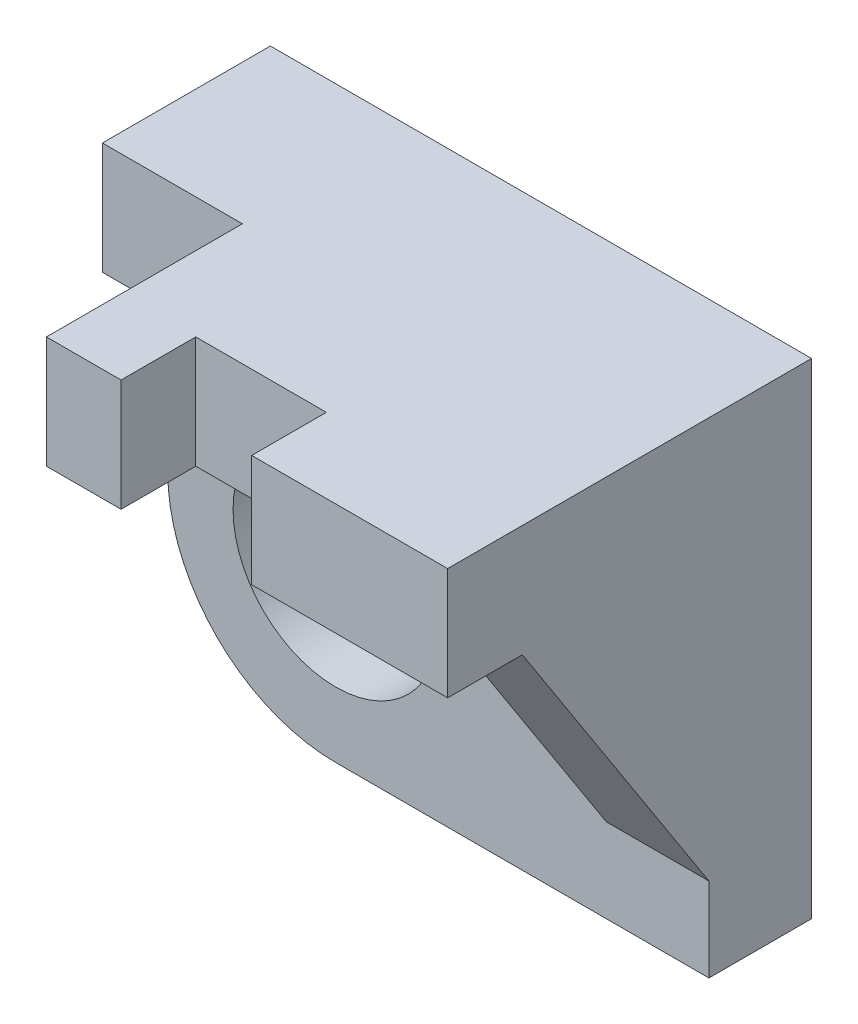
ISO-10303-21;
HEADER;
FILE_DESCRIPTION(('STEP AP214'),'2;1');
FILE_NAME('part.step','',(''),(''),'','','');
FILE_SCHEMA(('AUTOMOTIVE_DESIGN { 1 0 10303 214 1 1 1 1 }'));
ENDSEC;
DATA;
#1=APPLICATION_CONTEXT('core data for automotive mechanical design processes');
#2=APPLICATION_PROTOCOL_DEFINITION('international standard','automotive_design',2000,#1);
#3=PRODUCT_CONTEXT('',#1,'mechanical');
#4=PRODUCT('Part','Part','',(#3));
#5=PRODUCT_RELATED_PRODUCT_CATEGORY('part','',(#4));
#6=PRODUCT_DEFINITION_FORMATION('','',#4);
#7=PRODUCT_DEFINITION_CONTEXT('part definition',#1,'design');
#8=PRODUCT_DEFINITION('design','',#6,#7);
#9=PRODUCT_DEFINITION_SHAPE('','',#8);
#10=(LENGTH_UNIT() NAMED_UNIT(*) SI_UNIT(.MILLI.,.METRE.));
#11=(NAMED_UNIT(*) PLANE_ANGLE_UNIT() SI_UNIT($,.RADIAN.));
#12=(NAMED_UNIT(*) SI_UNIT($,.STERADIAN.) SOLID_ANGLE_UNIT());
#13=UNCERTAINTY_MEASURE_WITH_UNIT(LENGTH_MEASURE(1.E-05),#10,'distance_accuracy_value','');
#14=(GEOMETRIC_REPRESENTATION_CONTEXT(3) GLOBAL_UNCERTAINTY_ASSIGNED_CONTEXT((#13)) GLOBAL_UNIT_ASSIGNED_CONTEXT((#10,
#11,#12)) REPRESENTATION_CONTEXT('',''));
#15=CARTESIAN_POINT('',(0.,0.,0.));
#16=DIRECTION('',(0.,0.,1.));
#17=DIRECTION('',(1.,0.,0.));
#18=AXIS2_PLACEMENT_3D('',#15,#16,#17);
#19=CARTESIAN_POINT('',(18.,-34.,11.));
#20=DIRECTION('',(0.,0.,1.));
#21=DIRECTION('',(1.,0.,0.));
#22=AXIS2_PLACEMENT_3D('',#19,#20,#21);
#23=PLANE('',#22);
#24=CARTESIAN_POINT('',(18.,-34.,11.));
#25=DIRECTION('',(0.,0.,1.));
#26=DIRECTION('',(1.,0.,0.));
#27=AXIS2_PLACEMENT_3D('',#24,#25,#26);
#28=CIRCLE('',#27,11.);
#29=CARTESIAN_POINT('',(29.,-34.,11.));
#30=VERTEX_POINT('',#29);
#31=EDGE_CURVE('E287',#30,#30,#28,.T.);
#32=ORIENTED_EDGE('',*,*,#31,.F.);
#33=EDGE_LOOP('',(#32));
#34=FACE_BOUND('',#33,.T.);
#35=DIRECTION('',(1.,0.,0.));
#36=VECTOR('',#35,1.);
#37=CARTESIAN_POINT('',(47.,-43.,11.));
#38=LINE('',#37,#36);
#39=CARTESIAN_POINT('',(47.,-43.,11.));
#40=VERTEX_POINT('',#39);
#41=CARTESIAN_POINT('',(58.,-43.,11.));
#42=VERTEX_POINT('',#41);
#43=EDGE_CURVE('E168',#40,#42,#38,.T.);
#44=ORIENTED_EDGE('',*,*,#43,.F.);
#45=DIRECTION('',(0.,1.,0.));
#46=VECTOR('',#45,1.);
#47=CARTESIAN_POINT('',(47.,-12.,11.));
#48=LINE('',#47,#46);
#49=CARTESIAN_POINT('',(47.,-12.,11.));
#50=VERTEX_POINT('',#49);
#51=EDGE_CURVE('E162',#40,#50,#48,.T.);
#52=ORIENTED_EDGE('',*,*,#51,.T.);
#53=DIRECTION('',(-1.,0.,0.));
#54=VECTOR('',#53,1.);
#55=CARTESIAN_POINT('',(58.,-12.,11.));
#56=LINE('',#55,#54);
#57=CARTESIAN_POINT('',(0.,-12.,11.));
#58=VERTEX_POINT('',#57);
#59=EDGE_CURVE('E58',#50,#58,#56,.T.);
#60=ORIENTED_EDGE('',*,*,#59,.T.);
#61=DIRECTION('',(0.,-1.,0.));
#62=VECTOR('',#61,1.);
#63=CARTESIAN_POINT('',(0.,0.,11.));
#64=LINE('',#63,#62);
#65=CARTESIAN_POINT('',(0.,-34.,11.));
#66=VERTEX_POINT('',#65);
#67=EDGE_CURVE('E92',#58,#66,#64,.T.);
#68=ORIENTED_EDGE('',*,*,#67,.T.);
#69=CARTESIAN_POINT('',(18.,-34.,11.));
#70=DIRECTION('',(0.,0.,1.));
#71=DIRECTION('',(1.,0.,0.));
#72=AXIS2_PLACEMENT_3D('',#69,#70,#71);
#73=CIRCLE('',#72,18.);
#74=CARTESIAN_POINT('',(18.,-52.,11.));
#75=VERTEX_POINT('',#74);
#76=EDGE_CURVE('E248',#66,#75,#73,.T.);
#77=ORIENTED_EDGE('',*,*,#76,.T.);
#78=DIRECTION('',(1.,0.,0.));
#79=VECTOR('',#78,1.);
#80=CARTESIAN_POINT('',(58.,-52.,11.));
#81=LINE('',#80,#79);
#82=CARTESIAN_POINT('',(58.,-52.,11.));
#83=VERTEX_POINT('',#82);
#84=EDGE_CURVE('E68',#75,#83,#81,.T.);
#85=ORIENTED_EDGE('',*,*,#84,.T.);
#86=DIRECTION('',(0.,1.,0.));
#87=VECTOR('',#86,1.);
#88=CARTESIAN_POINT('',(58.,0.,11.));
#89=LINE('',#88,#87);
#90=EDGE_CURVE('E253',#83,#42,#89,.T.);
#91=ORIENTED_EDGE('',*,*,#90,.T.);
#92=EDGE_LOOP('',(#44,#52,#60,#68,#77,#85,#91));
#93=FACE_BOUND('',#92,.T.);
#94=ADVANCED_FACE('F44',(#34,#93),#23,.T.);
#95=CARTESIAN_POINT('',(0.,0.,11.));
#96=DIRECTION('',(0.,-1.,0.));
#97=DIRECTION('',(0.,0.,-1.));
#98=AXIS2_PLACEMENT_3D('',#95,#96,#97);
#99=PLANE('',#98);
#100=DIRECTION('',(-1.,0.,0.));
#101=VECTOR('',#100,1.);
#102=CARTESIAN_POINT('',(0.,0.,0.));
#103=LINE('',#102,#101);
#104=CARTESIAN_POINT('',(58.,0.,0.));
#105=VERTEX_POINT('',#104);
#106=CARTESIAN_POINT('',(0.,0.,0.));
#107=VERTEX_POINT('',#106);
#108=EDGE_CURVE('E235',#105,#107,#103,.T.);
#109=ORIENTED_EDGE('',*,*,#108,.T.);
#110=DIRECTION('',(0.,0.,-1.));
#111=VECTOR('',#110,1.);
#112=CARTESIAN_POINT('',(0.,0.,11.));
#113=LINE('',#112,#111);
#114=CARTESIAN_POINT('',(0.,0.,18.));
#115=VERTEX_POINT('',#114);
#116=EDGE_CURVE('E11',#115,#107,#113,.T.);
#117=ORIENTED_EDGE('',*,*,#116,.F.);
#118=DIRECTION('',(1.,0.,0.));
#119=VECTOR('',#118,1.);
#120=CARTESIAN_POINT('',(0.,0.,18.));
#121=LINE('',#120,#119);
#122=CARTESIAN_POINT('',(15.,0.,18.));
#123=VERTEX_POINT('',#122);
#124=EDGE_CURVE('E215',#115,#123,#121,.T.);
#125=ORIENTED_EDGE('',*,*,#124,.T.);
#126=DIRECTION('',(0.,0.,1.));
#127=VECTOR('',#126,1.);
#128=CARTESIAN_POINT('',(15.,0.,18.));
#129=LINE('',#128,#127);
#130=CARTESIAN_POINT('',(15.,0.,39.));
#131=VERTEX_POINT('',#130);
#132=EDGE_CURVE('E214',#123,#131,#129,.T.);
#133=ORIENTED_EDGE('',*,*,#132,.T.);
#134=DIRECTION('',(1.,0.,0.));
#135=VECTOR('',#134,1.);
#136=CARTESIAN_POINT('',(15.,0.,39.));
#137=LINE('',#136,#135);
#138=CARTESIAN_POINT('',(23.,0.,39.));
#139=VERTEX_POINT('',#138);
#140=EDGE_CURVE('E217',#131,#139,#137,.T.);
#141=ORIENTED_EDGE('',*,*,#140,.T.);
#142=DIRECTION('',(0.,0.,-1.));
#143=VECTOR('',#142,1.);
#144=CARTESIAN_POINT('',(23.,0.,39.));
#145=LINE('',#144,#143);
#146=CARTESIAN_POINT('',(23.,0.,31.));
#147=VERTEX_POINT('',#146);
#148=EDGE_CURVE('E222',#139,#147,#145,.T.);
#149=ORIENTED_EDGE('',*,*,#148,.T.);
#150=DIRECTION('',(1.,0.,0.));
#151=VECTOR('',#150,1.);
#152=CARTESIAN_POINT('',(37.,0.,31.));
#153=LINE('',#152,#151);
#154=CARTESIAN_POINT('',(37.,0.,31.));
#155=VERTEX_POINT('',#154);
#156=EDGE_CURVE('E221',#147,#155,#153,.T.);
#157=ORIENTED_EDGE('',*,*,#156,.T.);
#158=DIRECTION('',(0.,0.,1.));
#159=VECTOR('',#158,1.);
#160=CARTESIAN_POINT('',(37.,0.,39.));
#161=LINE('',#160,#159);
#162=CARTESIAN_POINT('',(37.,0.,39.));
#163=VERTEX_POINT('',#162);
#164=EDGE_CURVE('E185',#155,#163,#161,.T.);
#165=ORIENTED_EDGE('',*,*,#164,.T.);
#166=DIRECTION('',(1.,0.,0.));
#167=VECTOR('',#166,1.);
#168=CARTESIAN_POINT('',(58.,0.,39.));
#169=LINE('',#168,#167);
#170=CARTESIAN_POINT('',(58.,0.,39.));
#171=VERTEX_POINT('',#170);
#172=EDGE_CURVE('E180',#163,#171,#169,.T.);
#173=ORIENTED_EDGE('',*,*,#172,.T.);
#174=DIRECTION('',(0.,0.,-1.));
#175=VECTOR('',#174,1.);
#176=CARTESIAN_POINT('',(58.,0.,11.));
#177=LINE('',#176,#175);
#178=EDGE_CURVE('E251',#171,#105,#177,.T.);
#179=ORIENTED_EDGE('',*,*,#178,.T.);
#180=EDGE_LOOP('',(#109,#117,#125,#133,#141,#149,#157,#165,#173,#179));
#181=FACE_BOUND('',#180,.T.);
#182=ADVANCED_FACE('F50',(#181),#99,.F.);
#183=CARTESIAN_POINT('',(0.,0.,11.));
#184=DIRECTION('',(1.,0.,0.));
#185=DIRECTION('',(0.,0.,-1.));
#186=AXIS2_PLACEMENT_3D('',#183,#184,#185);
#187=PLANE('',#186);
#188=DIRECTION('',(0.,-1.,0.));
#189=VECTOR('',#188,1.);
#190=CARTESIAN_POINT('',(0.,0.,0.));
#191=LINE('',#190,#189);
#192=CARTESIAN_POINT('',(0.,-34.,0.));
#193=VERTEX_POINT('',#192);
#194=EDGE_CURVE('E258',#107,#193,#191,.T.);
#195=ORIENTED_EDGE('',*,*,#194,.T.);
#196=DIRECTION('',(0.,0.,-1.));
#197=VECTOR('',#196,1.);
#198=CARTESIAN_POINT('',(0.,-34.,11.));
#199=LINE('',#198,#197);
#200=EDGE_CURVE('E52',#66,#193,#199,.T.);
#201=ORIENTED_EDGE('',*,*,#200,.F.);
#202=ORIENTED_EDGE('',*,*,#67,.F.);
#203=DIRECTION('',(0.,0.,1.));
#204=VECTOR('',#203,1.);
#205=CARTESIAN_POINT('',(0.,-12.,11.));
#206=LINE('',#205,#204);
#207=CARTESIAN_POINT('',(0.,-12.,18.));
#208=VERTEX_POINT('',#207);
#209=EDGE_CURVE('E176',#58,#208,#206,.T.);
#210=ORIENTED_EDGE('',*,*,#209,.T.);
#211=DIRECTION('',(0.,1.,0.));
#212=VECTOR('',#211,1.);
#213=CARTESIAN_POINT('',(0.,-12.,18.));
#214=LINE('',#213,#212);
#215=EDGE_CURVE('E211',#208,#115,#214,.T.);
#216=ORIENTED_EDGE('',*,*,#215,.T.);
#217=ORIENTED_EDGE('',*,*,#116,.T.);
#218=EDGE_LOOP('',(#195,#201,#202,#210,#216,#217));
#219=FACE_BOUND('',#218,.T.);
#220=ADVANCED_FACE('F310',(#219),#187,.F.);
#221=CARTESIAN_POINT('',(18.,-34.,11.));
#222=DIRECTION('',(0.,0.,-1.));
#223=DIRECTION('',(-1.,0.,0.));
#224=AXIS2_PLACEMENT_3D('',#221,#222,#223);
#225=CYLINDRICAL_SURFACE('',#224,18.);
#226=CARTESIAN_POINT('',(18.,-34.,0.));
#227=DIRECTION('',(0.,0.,1.));
#228=DIRECTION('',(1.,0.,0.));
#229=AXIS2_PLACEMENT_3D('',#226,#227,#228);
#230=CIRCLE('',#229,18.);
#231=CARTESIAN_POINT('',(18.,-52.,0.));
#232=VERTEX_POINT('',#231);
#233=EDGE_CURVE('E256',#193,#232,#230,.T.);
#234=ORIENTED_EDGE('',*,*,#233,.T.);
#235=DIRECTION('',(0.,0.,-1.));
#236=VECTOR('',#235,1.);
#237=CARTESIAN_POINT('',(18.,-52.,11.));
#238=LINE('',#237,#236);
#239=EDGE_CURVE('E266',#75,#232,#238,.T.);
#240=ORIENTED_EDGE('',*,*,#239,.F.);
#241=ORIENTED_EDGE('',*,*,#76,.F.);
#242=ORIENTED_EDGE('',*,*,#200,.T.);
#243=EDGE_LOOP('',(#234,#240,#241,#242));
#244=FACE_BOUND('',#243,.T.);
#245=ADVANCED_FACE('F275',(#244),#225,.T.);
#246=CARTESIAN_POINT('',(58.,-52.,11.));
#247=DIRECTION('',(0.,1.,0.));
#248=DIRECTION('',(-1.,0.,0.));
#249=AXIS2_PLACEMENT_3D('',#246,#247,#248);
#250=PLANE('',#249);
#251=DIRECTION('',(1.,0.,0.));
#252=VECTOR('',#251,1.);
#253=CARTESIAN_POINT('',(58.,-52.,0.));
#254=LINE('',#253,#252);
#255=CARTESIAN_POINT('',(58.,-52.,0.));
#256=VERTEX_POINT('',#255);
#257=EDGE_CURVE('E257',#232,#256,#254,.T.);
#258=ORIENTED_EDGE('',*,*,#257,.T.);
#259=DIRECTION('',(0.,0.,-1.));
#260=VECTOR('',#259,1.);
#261=CARTESIAN_POINT('',(58.,-52.,11.));
#262=LINE('',#261,#260);
#263=EDGE_CURVE('E262',#83,#256,#262,.T.);
#264=ORIENTED_EDGE('',*,*,#263,.F.);
#265=ORIENTED_EDGE('',*,*,#84,.F.);
#266=ORIENTED_EDGE('',*,*,#239,.T.);
#267=EDGE_LOOP('',(#258,#264,#265,#266));
#268=FACE_BOUND('',#267,.T.);
#269=ADVANCED_FACE('F278',(#268),#250,.F.);
#270=CARTESIAN_POINT('',(58.,0.,11.));
#271=DIRECTION('',(-1.,0.,0.));
#272=DIRECTION('',(0.,0.,1.));
#273=AXIS2_PLACEMENT_3D('',#270,#271,#272);
#274=PLANE('',#273);
#275=DIRECTION('',(0.,1.,0.));
#276=VECTOR('',#275,1.);
#277=CARTESIAN_POINT('',(58.,0.,0.));
#278=LINE('',#277,#276);
#279=EDGE_CURVE('E95',#256,#105,#278,.T.);
#280=ORIENTED_EDGE('',*,*,#279,.T.);
#281=ORIENTED_EDGE('',*,*,#178,.F.);
#282=DIRECTION('',(0.,1.,0.));
#283=VECTOR('',#282,1.);
#284=CARTESIAN_POINT('',(58.,-12.,39.));
#285=LINE('',#284,#283);
#286=CARTESIAN_POINT('',(58.,-12.,39.));
#287=VERTEX_POINT('',#286);
#288=EDGE_CURVE('E229',#287,#171,#285,.T.);
#289=ORIENTED_EDGE('',*,*,#288,.F.);
#290=DIRECTION('',(0.,0.,-1.));
#291=VECTOR('',#290,1.);
#292=CARTESIAN_POINT('',(58.,-12.,11.));
#293=LINE('',#292,#291);
#294=CARTESIAN_POINT('',(58.,-12.,31.));
#295=VERTEX_POINT('',#294);
#296=EDGE_CURVE('E208',#287,#295,#293,.T.);
#297=ORIENTED_EDGE('',*,*,#296,.T.);
#298=DIRECTION('',(0.,-0.840296648224244,-0.542126869822093));
#299=VECTOR('',#298,1.);
#300=CARTESIAN_POINT('',(58.,-43.,11.));
#301=LINE('',#300,#299);
#302=EDGE_CURVE('E172',#295,#42,#301,.T.);
#303=ORIENTED_EDGE('',*,*,#302,.T.);
#304=ORIENTED_EDGE('',*,*,#90,.F.);
#305=ORIENTED_EDGE('',*,*,#263,.T.);
#306=EDGE_LOOP('',(#280,#281,#289,#297,#303,#304,#305));
#307=FACE_BOUND('',#306,.T.);
#308=ADVANCED_FACE('F285',(#307),#274,.F.);
#309=CARTESIAN_POINT('',(18.,-34.,0.));
#310=DIRECTION('',(0.,0.,1.));
#311=DIRECTION('',(1.,0.,0.));
#312=AXIS2_PLACEMENT_3D('',#309,#310,#311);
#313=PLANE('',#312);
#314=CARTESIAN_POINT('',(18.,-34.,0.));
#315=DIRECTION('',(0.,0.,1.));
#316=DIRECTION('',(1.,0.,0.));
#317=AXIS2_PLACEMENT_3D('',#314,#315,#316);
#318=CIRCLE('',#317,11.);
#319=CARTESIAN_POINT('',(29.,-34.,0.));
#320=VERTEX_POINT('',#319);
#321=EDGE_CURVE('E286',#320,#320,#318,.T.);
#322=ORIENTED_EDGE('',*,*,#321,.T.);
#323=EDGE_LOOP('',(#322));
#324=FACE_BOUND('',#323,.T.);
#325=ORIENTED_EDGE('',*,*,#108,.F.);
#326=ORIENTED_EDGE('',*,*,#279,.F.);
#327=ORIENTED_EDGE('',*,*,#257,.F.);
#328=ORIENTED_EDGE('',*,*,#233,.F.);
#329=ORIENTED_EDGE('',*,*,#194,.F.);
#330=EDGE_LOOP('',(#325,#326,#327,#328,#329));
#331=FACE_BOUND('',#330,.T.);
#332=ADVANCED_FACE('F279',(#324,#331),#313,.F.);
#333=CARTESIAN_POINT('',(58.,-12.,39.));
#334=DIRECTION('',(0.,0.,1.));
#335=DIRECTION('',(1.,0.,0.));
#336=AXIS2_PLACEMENT_3D('',#333,#334,#335);
#337=PLANE('',#336);
#338=ORIENTED_EDGE('',*,*,#172,.F.);
#339=DIRECTION('',(0.,1.,0.));
#340=VECTOR('',#339,1.);
#341=CARTESIAN_POINT('',(37.,-12.,39.));
#342=LINE('',#341,#340);
#343=CARTESIAN_POINT('',(37.,-12.,39.));
#344=VERTEX_POINT('',#343);
#345=EDGE_CURVE('E233',#344,#163,#342,.T.);
#346=ORIENTED_EDGE('',*,*,#345,.F.);
#347=DIRECTION('',(1.,0.,0.));
#348=VECTOR('',#347,1.);
#349=CARTESIAN_POINT('',(58.,-12.,39.));
#350=LINE('',#349,#348);
#351=EDGE_CURVE('E202',#344,#287,#350,.T.);
#352=ORIENTED_EDGE('',*,*,#351,.T.);
#353=ORIENTED_EDGE('',*,*,#288,.T.);
#354=EDGE_LOOP('',(#338,#346,#352,#353));
#355=FACE_BOUND('',#354,.T.);
#356=ADVANCED_FACE('F320',(#355),#337,.T.);
#357=CARTESIAN_POINT('',(37.,-12.,39.));
#358=DIRECTION('',(-1.,0.,0.));
#359=DIRECTION('',(0.,0.,1.));
#360=AXIS2_PLACEMENT_3D('',#357,#358,#359);
#361=PLANE('',#360);
#362=ORIENTED_EDGE('',*,*,#164,.F.);
#363=DIRECTION('',(0.,1.,0.));
#364=VECTOR('',#363,1.);
#365=CARTESIAN_POINT('',(37.,-12.,31.));
#366=LINE('',#365,#364);
#367=CARTESIAN_POINT('',(37.,-12.,31.));
#368=VERTEX_POINT('',#367);
#369=EDGE_CURVE('E234',#368,#155,#366,.T.);
#370=ORIENTED_EDGE('',*,*,#369,.F.);
#371=DIRECTION('',(0.,0.,1.));
#372=VECTOR('',#371,1.);
#373=CARTESIAN_POINT('',(37.,-12.,39.));
#374=LINE('',#373,#372);
#375=EDGE_CURVE('E205',#368,#344,#374,.T.);
#376=ORIENTED_EDGE('',*,*,#375,.T.);
#377=ORIENTED_EDGE('',*,*,#345,.T.);
#378=EDGE_LOOP('',(#362,#370,#376,#377));
#379=FACE_BOUND('',#378,.T.);
#380=ADVANCED_FACE('F333',(#379),#361,.T.);
#381=CARTESIAN_POINT('',(37.,-12.,31.));
#382=DIRECTION('',(0.,0.,1.));
#383=DIRECTION('',(1.,0.,0.));
#384=AXIS2_PLACEMENT_3D('',#381,#382,#383);
#385=PLANE('',#384);
#386=ORIENTED_EDGE('',*,*,#156,.F.);
#387=DIRECTION('',(0.,1.,0.));
#388=VECTOR('',#387,1.);
#389=CARTESIAN_POINT('',(23.,-12.,31.));
#390=LINE('',#389,#388);
#391=CARTESIAN_POINT('',(23.,-12.,31.));
#392=VERTEX_POINT('',#391);
#393=EDGE_CURVE('E240',#392,#147,#390,.T.);
#394=ORIENTED_EDGE('',*,*,#393,.F.);
#395=DIRECTION('',(1.,0.,0.));
#396=VECTOR('',#395,1.);
#397=CARTESIAN_POINT('',(37.,-12.,31.));
#398=LINE('',#397,#396);
#399=EDGE_CURVE('E200',#392,#368,#398,.T.);
#400=ORIENTED_EDGE('',*,*,#399,.T.);
#401=ORIENTED_EDGE('',*,*,#369,.T.);
#402=EDGE_LOOP('',(#386,#394,#400,#401));
#403=FACE_BOUND('',#402,.T.);
#404=ADVANCED_FACE('F338',(#403),#385,.T.);
#405=CARTESIAN_POINT('',(23.,-12.,39.));
#406=DIRECTION('',(1.,0.,0.));
#407=DIRECTION('',(0.,0.,-1.));
#408=AXIS2_PLACEMENT_3D('',#405,#406,#407);
#409=PLANE('',#408);
#410=ORIENTED_EDGE('',*,*,#148,.F.);
#411=DIRECTION('',(0.,1.,0.));
#412=VECTOR('',#411,1.);
#413=CARTESIAN_POINT('',(23.,-12.,39.));
#414=LINE('',#413,#412);
#415=CARTESIAN_POINT('',(23.,-12.,39.));
#416=VERTEX_POINT('',#415);
#417=EDGE_CURVE('E239',#416,#139,#414,.T.);
#418=ORIENTED_EDGE('',*,*,#417,.F.);
#419=DIRECTION('',(0.,0.,-1.));
#420=VECTOR('',#419,1.);
#421=CARTESIAN_POINT('',(23.,-12.,39.));
#422=LINE('',#421,#420);
#423=EDGE_CURVE('E198',#416,#392,#422,.T.);
#424=ORIENTED_EDGE('',*,*,#423,.T.);
#425=ORIENTED_EDGE('',*,*,#393,.T.);
#426=EDGE_LOOP('',(#410,#418,#424,#425));
#427=FACE_BOUND('',#426,.T.);
#428=ADVANCED_FACE('F343',(#427),#409,.T.);
#429=CARTESIAN_POINT('',(15.,-12.,39.));
#430=DIRECTION('',(0.,0.,1.));
#431=DIRECTION('',(1.,0.,0.));
#432=AXIS2_PLACEMENT_3D('',#429,#430,#431);
#433=PLANE('',#432);
#434=ORIENTED_EDGE('',*,*,#140,.F.);
#435=DIRECTION('',(0.,1.,0.));
#436=VECTOR('',#435,1.);
#437=CARTESIAN_POINT('',(15.,-12.,39.));
#438=LINE('',#437,#436);
#439=CARTESIAN_POINT('',(15.,-12.,39.));
#440=VERTEX_POINT('',#439);
#441=EDGE_CURVE('E242',#440,#131,#438,.T.);
#442=ORIENTED_EDGE('',*,*,#441,.F.);
#443=DIRECTION('',(1.,0.,0.));
#444=VECTOR('',#443,1.);
#445=CARTESIAN_POINT('',(15.,-12.,39.));
#446=LINE('',#445,#444);
#447=EDGE_CURVE('E193',#440,#416,#446,.T.);
#448=ORIENTED_EDGE('',*,*,#447,.T.);
#449=ORIENTED_EDGE('',*,*,#417,.T.);
#450=EDGE_LOOP('',(#434,#442,#448,#449));
#451=FACE_BOUND('',#450,.T.);
#452=ADVANCED_FACE('F347',(#451),#433,.T.);
#453=CARTESIAN_POINT('',(15.,-12.,18.));
#454=DIRECTION('',(-1.,0.,0.));
#455=DIRECTION('',(0.,0.,1.));
#456=AXIS2_PLACEMENT_3D('',#453,#454,#455);
#457=PLANE('',#456);
#458=ORIENTED_EDGE('',*,*,#132,.F.);
#459=DIRECTION('',(0.,1.,0.));
#460=VECTOR('',#459,1.);
#461=CARTESIAN_POINT('',(15.,-12.,18.));
#462=LINE('',#461,#460);
#463=CARTESIAN_POINT('',(15.,-12.,18.));
#464=VERTEX_POINT('',#463);
#465=EDGE_CURVE('E243',#464,#123,#462,.T.);
#466=ORIENTED_EDGE('',*,*,#465,.F.);
#467=DIRECTION('',(0.,0.,1.));
#468=VECTOR('',#467,1.);
#469=CARTESIAN_POINT('',(15.,-12.,18.));
#470=LINE('',#469,#468);
#471=EDGE_CURVE('E186',#464,#440,#470,.T.);
#472=ORIENTED_EDGE('',*,*,#471,.T.);
#473=ORIENTED_EDGE('',*,*,#441,.T.);
#474=EDGE_LOOP('',(#458,#466,#472,#473));
#475=FACE_BOUND('',#474,.T.);
#476=ADVANCED_FACE('F348',(#475),#457,.T.);
#477=CARTESIAN_POINT('',(0.,-12.,18.));
#478=DIRECTION('',(0.,0.,1.));
#479=DIRECTION('',(1.,0.,0.));
#480=AXIS2_PLACEMENT_3D('',#477,#478,#479);
#481=PLANE('',#480);
#482=ORIENTED_EDGE('',*,*,#124,.F.);
#483=ORIENTED_EDGE('',*,*,#215,.F.);
#484=DIRECTION('',(1.,0.,0.));
#485=VECTOR('',#484,1.);
#486=CARTESIAN_POINT('',(0.,-12.,18.));
#487=LINE('',#486,#485);
#488=EDGE_CURVE('E177',#208,#464,#487,.T.);
#489=ORIENTED_EDGE('',*,*,#488,.T.);
#490=ORIENTED_EDGE('',*,*,#465,.T.);
#491=EDGE_LOOP('',(#482,#483,#489,#490));
#492=FACE_BOUND('',#491,.T.);
#493=ADVANCED_FACE('F301',(#492),#481,.T.);
#494=CARTESIAN_POINT('',(0.,-12.,0.));
#495=DIRECTION('',(0.,1.,0.));
#496=DIRECTION('',(0.,0.,1.));
#497=AXIS2_PLACEMENT_3D('',#494,#495,#496);
#498=PLANE('',#497);
#499=DIRECTION('',(0.,0.,1.));
#500=VECTOR('',#499,1.);
#501=CARTESIAN_POINT('',(47.,-12.,11.));
#502=LINE('',#501,#500);
#503=CARTESIAN_POINT('',(47.,-12.,31.));
#504=VERTEX_POINT('',#503);
#505=EDGE_CURVE('E161',#50,#504,#502,.T.);
#506=ORIENTED_EDGE('',*,*,#505,.T.);
#507=DIRECTION('',(1.,0.,0.));
#508=VECTOR('',#507,1.);
#509=CARTESIAN_POINT('',(47.,-12.,31.));
#510=LINE('',#509,#508);
#511=EDGE_CURVE('E183',#504,#295,#510,.T.);
#512=ORIENTED_EDGE('',*,*,#511,.T.);
#513=ORIENTED_EDGE('',*,*,#296,.F.);
#514=ORIENTED_EDGE('',*,*,#351,.F.);
#515=ORIENTED_EDGE('',*,*,#375,.F.);
#516=ORIENTED_EDGE('',*,*,#399,.F.);
#517=ORIENTED_EDGE('',*,*,#423,.F.);
#518=ORIENTED_EDGE('',*,*,#447,.F.);
#519=ORIENTED_EDGE('',*,*,#471,.F.);
#520=ORIENTED_EDGE('',*,*,#488,.F.);
#521=ORIENTED_EDGE('',*,*,#209,.F.);
#522=ORIENTED_EDGE('',*,*,#59,.F.);
#523=EDGE_LOOP('',(#506,#512,#513,#514,#515,#516,#517,#518,#519,#520,#521,#522));
#524=FACE_BOUND('',#523,.T.);
#525=ADVANCED_FACE('F173',(#524),#498,.F.);
#526=CARTESIAN_POINT('',(47.,-43.,11.));
#527=DIRECTION('',(0.,-0.542126869822093,0.840296648224244));
#528=DIRECTION('',(0.,-0.840296648224244,-0.542126869822093));
#529=AXIS2_PLACEMENT_3D('',#526,#527,#528);
#530=PLANE('',#529);
#531=ORIENTED_EDGE('',*,*,#302,.F.);
#532=ORIENTED_EDGE('',*,*,#511,.F.);
#533=DIRECTION('',(0.,-0.840296648224244,-0.542126869822093));
#534=VECTOR('',#533,1.);
#535=CARTESIAN_POINT('',(47.,-43.,11.));
#536=LINE('',#535,#534);
#537=EDGE_CURVE('E164',#504,#40,#536,.T.);
#538=ORIENTED_EDGE('',*,*,#537,.T.);
#539=ORIENTED_EDGE('',*,*,#43,.T.);
#540=EDGE_LOOP('',(#531,#532,#538,#539));
#541=FACE_BOUND('',#540,.T.);
#542=ADVANCED_FACE('F295',(#541),#530,.T.);
#543=CARTESIAN_POINT('',(47.,0.,0.));
#544=DIRECTION('',(-1.,0.,0.));
#545=DIRECTION('',(0.,0.,1.));
#546=AXIS2_PLACEMENT_3D('',#543,#544,#545);
#547=PLANE('',#546);
#548=ORIENTED_EDGE('',*,*,#51,.F.);
#549=ORIENTED_EDGE('',*,*,#537,.F.);
#550=ORIENTED_EDGE('',*,*,#505,.F.);
#551=EDGE_LOOP('',(#548,#549,#550));
#552=FACE_BOUND('',#551,.T.);
#553=ADVANCED_FACE('F165',(#552),#547,.T.);
#554=CARTESIAN_POINT('',(18.,-34.,0.));
#555=DIRECTION('',(0.,0.,1.));
#556=DIRECTION('',(1.,0.,0.));
#557=AXIS2_PLACEMENT_3D('',#554,#555,#556);
#558=CYLINDRICAL_SURFACE('',#557,11.);
#559=ORIENTED_EDGE('',*,*,#321,.F.);
#560=EDGE_LOOP('',(#559));
#561=FACE_BOUND('',#560,.T.);
#562=ORIENTED_EDGE('',*,*,#31,.T.);
#563=EDGE_LOOP('',(#562));
#564=FACE_BOUND('',#563,.T.);
#565=ADVANCED_FACE('F299',(#561,#564),#558,.F.);
#566=CLOSED_SHELL('',(#94,#182,#220,#245,#269,#308,#332,#356,#380,#404,#428,#452,#476,#493,#525,
#542,#553,#565));
#567=MANIFOLD_SOLID_BREP('B2',#566);
#568=ADVANCED_BREP_SHAPE_REPRESENTATION('',(#18,#567),#14);
#569=SHAPE_DEFINITION_REPRESENTATION(#9,#568);
ENDSEC;
END-ISO-10303-21;
